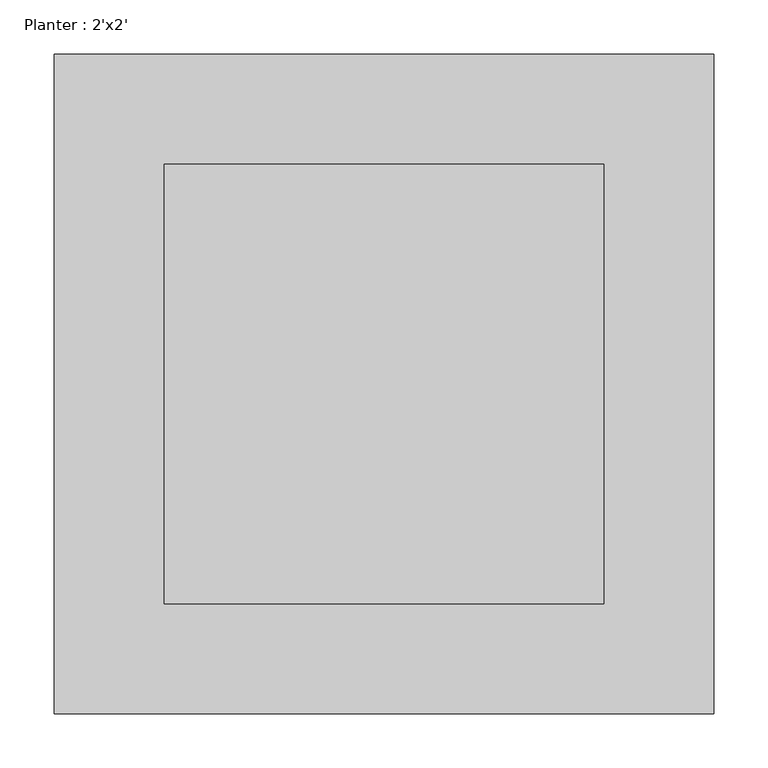
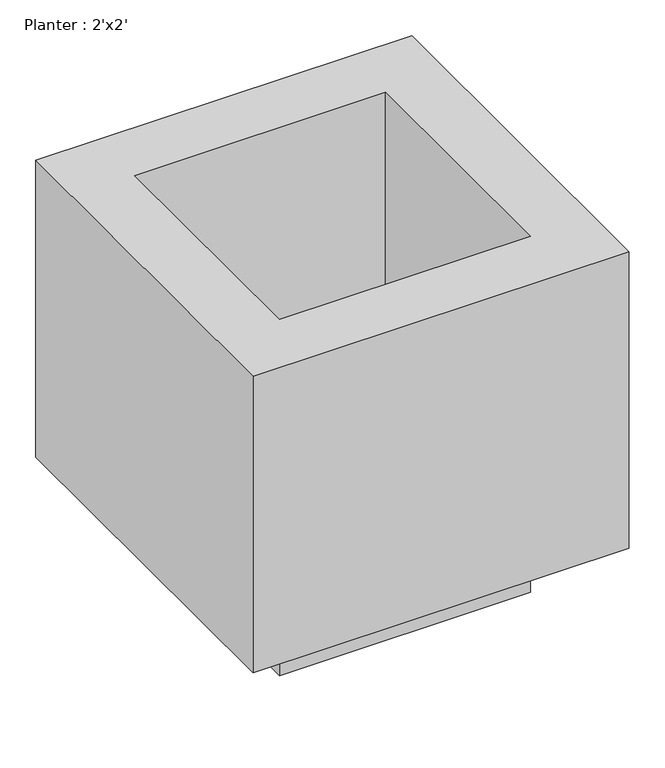
"""IFC4 building model written with IfcOpenShell, lengths in millimetres: geographic element geometry, Planter : 2'x2'."""

from ifc_helpers import new_model, si_unit, origin, origin_with_axes, place, context, project, spatial, polyline, outline, extrude, faceted_brep, source, transform, mapped, element, save


def planter_2_x2_da431093(model_context):
    return source(origin(), model_context, "Body", "SolidModel", [
        faceted_brep([(304.8, 304.8, 609.6), (-304.8, 304.8, 609.6), (-304.8, -304.8, 609.6), (304.8, -304.8, 609.6), (-203.2, 203.2, 609.6), (203.2, 203.2, 609.6), (203.2, -203.2, 609.6), (-203.2, -203.2, 609.6), (304.8, 304.8, 101.6), (304.8, -304.8, 101.6), (-304.8, -304.8, 101.6), (-304.8, 304.8, 101.6), (203.2, 203.2, 203.2), (-203.2, 203.2, 203.2), (-203.2, -203.2, 203.2), (203.2, -203.2, 203.2)], [[[0, 1, 2, 3], [4, 5, 6, 7]], [[8, 9, 10, 11]], [[1, 0, 8, 11]], [[2, 1, 11, 10]], [[3, 2, 10, 9]], [[0, 3, 9, 8]], [[12, 13, 14, 15]], [[13, 12, 5, 4]], [[14, 13, 4, 7]], [[15, 14, 7, 6]], [[12, 15, 6, 5]]]),
        extrude(outline(polyline([(203.2, 203.2), (203.2, -203.2), (-203.2, -203.2), (-203.2, 203.2), (203.2, 203.2)])), origin_with_axes(), (0.0, 0.0, 1.0), 101.6),
    ])


if __name__ == "__main__":
    model = new_model("IFC4")
    model_context = context("Model", 3, world=origin())
    ifc_project = project(units=[si_unit("LENGTHUNIT", "METRE", prefix="MILLI")], contexts=[model_context])
    site = spatial("IfcSite", under=ifc_project)
    building = spatial("IfcBuilding", under=site)
    placement = place(None, origin())
    planter_2_x2_shape = planter_2_x2_da431093(model_context)
    element("IfcGeographicElement", 1, ObjectType="Planter : 2'x2'", at=placement, inside=building, context=model_context, shape_type="MappedRepresentation", body=[
        mapped(planter_2_x2_shape, transform((0.0, 0.0, 0.0), x_axis=(1.0, 0.0, 0.0), y_axis=(0.0, 1.0, 0.0), z_axis=(0.0, 0.0, 1.0))),
    ])
    save(model, "model.ifc")

# Revit data of these elements
# Type "Planter : 2'x2'"
#   Depth = 2' - 0"
#   Height = 2' - 0"
#   Width = 2' - 0"
#   Material = Concrete, Precast
# Element 1 (IfcGeographicElement, "Planter : 2'x2'")
#   Materials on its faces: "Concrete, Precast"
# Materials
#   "Concrete, Precast": class "Concrete", colour RGB 198 187 187, transparency 0, Description = "Precast concrete", Cost = 0
